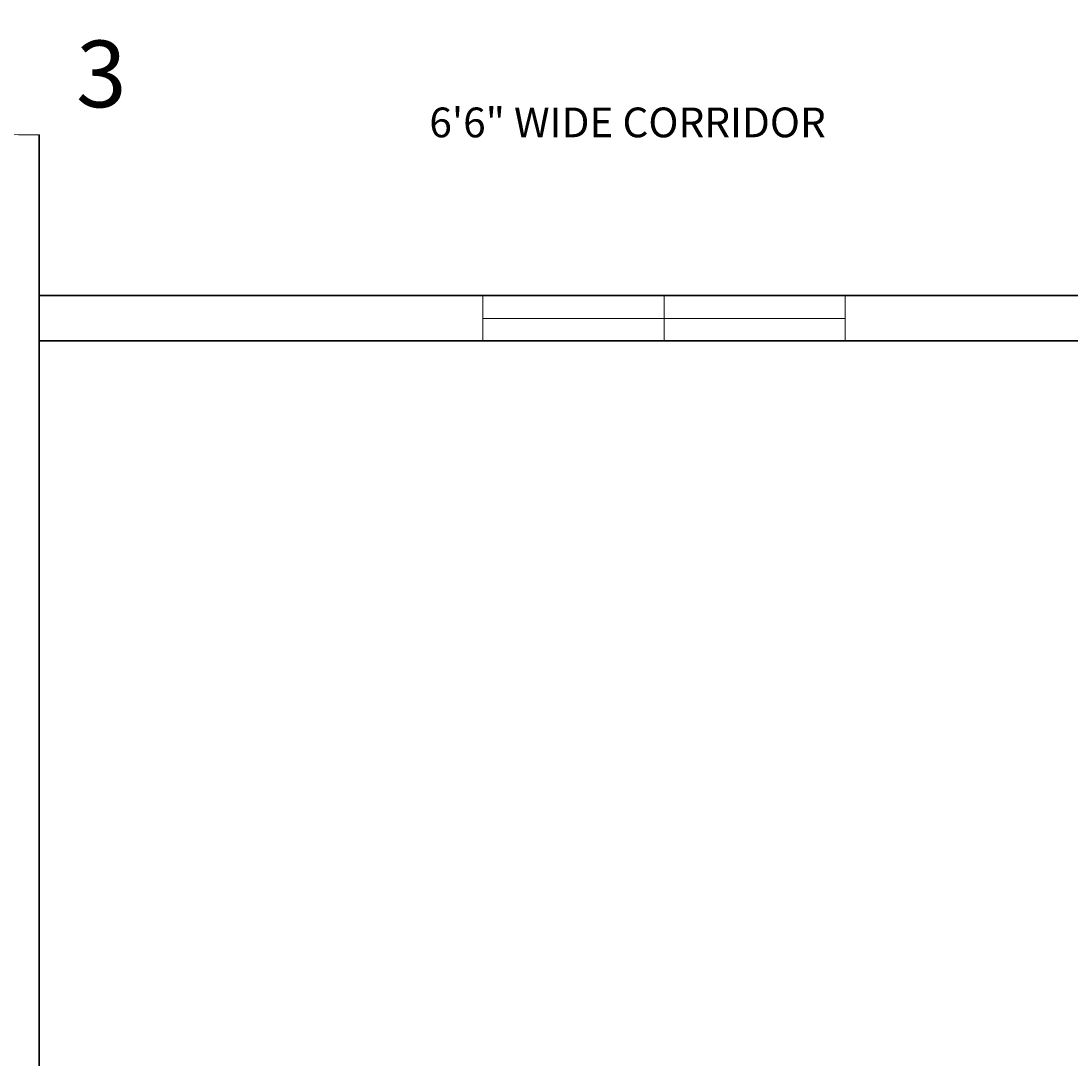
# Model space of a CAD drawing. Units: millimetres. Extents: x 27017497 to 27018854, y 7058029 to 7059154.
# Tile 59 of 91: x 27018038 to 27018246, y 7058203 to 7058409. Entities that reach past the tile are written whole.
import ezdxf

# ---------------------------------------------------------------- set-up
doc = ezdxf.new("R2010")
doc.units = ezdxf.units.MM
for name, color, linetype, lineweight in [('A-ANNO-DIMS', 2, 'Continuous', 18), ('A-ANNO-IDEN', 7, 'Continuous', 18), ('A-AREA-IDEN', 7, 'Continuous', 18), ('A-DOOR', 4, 'Continuous', 20), ('A-GLAZ', 4, 'Continuous', 18), ('A-WALL', 7, 'Continuous', 35)]:
    doc.layers.add(name, color=color, linetype=linetype, lineweight=lineweight)
doc.styles.get("Standard").update_dxf_attribs({"font": 'arial.ttf'})
doc.dimstyles.get("Standard").update_dxf_attribs({"dimtxt": 0.18, "dimasz": 0.18, "dimexe": 0.18, "dimexo": 0.0625, "dimgap": 0.09, "dimtad": 0, "dimtih": 1, "dimtoh": 1, "dimdec": 4, "dimzin": 0, "dimdsep": 46, "dimtxsty": 'Standard', "dimcen": 0.09, "dimadec": 0, "dimazin": 0, "dimtfac": 1, "dimtdec": 4, "dimtofl": 0, "dimtmove": 0, "dimatfit": 3, "dimfxl": 1, "dimtolj": 1, "dimtzin": 0, "dimarcsym": 0})

# ---------------------------------------------------------------- blocks, each defined once
blk = doc.blocks.new('*U2')
for p, q in [((0, 0), (0, -6)), ((40, 0), (40, -6))]:
    blk.add_line(p, q)
blk.add_lwpolyline([(0, 0), (0, 40), (1.75, 40), (1.75, 0)], close=True)
blk.add_arc((0, 0), 40, 0, 90)
blk = doc.blocks.new('WINDOW-SINGLE-LIGHT')
blk.add_lwpolyline([(36, 4.5), (36, 0), (0, 0), (0, 9), (36, 9), (36, 4.5), (0, 4.5)])
blk = doc.blocks.new('*D47')
at = {"layer": 'A-ANNO-DIMS', "color": 0, "lineweight": -2, "transparency": 16777216}
for p, q in [((27017561.17, 7058294.35), (27017561.17, 7058028.6)), ((27018790.61, 7058294.35), (27018790.61, 7058028.6)), ((27017561.35, 7058028.78), (27018175.43, 7058028.78)), ((27018790.43, 7058028.78), (27018176.34, 7058028.78))]:
    blk.add_line(p, q, dxfattribs=at)
at = {"layer": 'A-ANNO-DIMS', "color": 0, "transparency": 16777216}
for points in [[(27017561.35, 7058028.81), (27017561.35, 7058028.75), (27017561.17, 7058028.78)], [(27018790.43, 7058028.81), (27018790.43, 7058028.75), (27018790.61, 7058028.78)]]:
    blk.add_solid(points, dxfattribs=at)
at = {"layer": 'Defpoints', "color": 0, "transparency": 16777216}
for p in [(27017561.17, 7058294.41), (27018790.61, 7058294.41), (27018790.61, 7058028.78)]:
    blk.add_point(p, dxfattribs=at)
at = {"layer": 'A-ANNO-DIMS', "color": 0, "transparency": 16777216, "insert": (27018175.89, 7058028.78), "char_height": 0.18, "attachment_point": 5}
blk.add_mtext('\\A1;1229.4', dxfattribs=at)
blk = doc.blocks.new('*D48')
at = {"layer": 'A-ANNO-DIMS', "color": 0, "lineweight": -2, "transparency": 16777216}
for p, q in [((27018463.5, 7058622.91), (27017497.54, 7058622.91)), ((27017497.72, 7058622.73), (27017497.72, 7058357.75)), ((27017497.72, 7058092.41), (27017497.72, 7058357.39)), ((27018555.13, 7058092.23), (27017497.54, 7058092.23))]:
    blk.add_line(p, q, dxfattribs=at)
at = {"layer": 'A-ANNO-DIMS', "color": 0, "transparency": 16777216}
for points in [[(27017497.69, 7058622.73), (27017497.75, 7058622.73), (27017497.72, 7058622.91)], [(27017497.69, 7058092.41), (27017497.75, 7058092.41), (27017497.72, 7058092.23)]]:
    blk.add_solid(points, dxfattribs=at)
at = {"layer": 'Defpoints', "color": 0, "transparency": 16777216}
for p in [(27018463.56, 7058622.91), (27017497.72, 7058092.23), (27018555.19, 7058092.23)]:
    blk.add_point(p, dxfattribs=at)
at = {"layer": 'A-ANNO-DIMS', "color": 0, "transparency": 16777216, "insert": (27017497.72, 7058357.57), "char_height": 0.18, "attachment_point": 5}
blk.add_mtext('\\A1;530.7', dxfattribs=at)
blk = doc.blocks.new('*D51')
at = {"layer": 'A-ANNO-DIMS', "color": 0, "lineweight": -2, "transparency": 16777216}
for p, q in [((27018041.17, 7058345.35), (27018041.17, 7058028.6)), ((27018310.61, 7058345.35), (27018310.61, 7058028.6)), ((27018041.35, 7058028.78), (27018175.42, 7058028.78)), ((27018310.43, 7058028.78), (27018176.35, 7058028.78))]:
    blk.add_line(p, q, dxfattribs=at)
at = {"layer": 'A-ANNO-DIMS', "color": 0, "transparency": 16777216}
for points in [[(27018041.35, 7058028.81), (27018041.35, 7058028.75), (27018041.17, 7058028.78)], [(27018310.43, 7058028.81), (27018310.43, 7058028.75), (27018310.61, 7058028.78)]]:
    blk.add_solid(points, dxfattribs=at)
at = {"layer": 'Defpoints', "color": 0, "transparency": 16777216}
for p in [(27018041.17, 7058345.41), (27018310.61, 7058345.41), (27018310.61, 7058028.78)]:
    blk.add_point(p, dxfattribs=at)
at = {"layer": 'A-ANNO-DIMS', "color": 0, "transparency": 16777216, "insert": (27018175.89, 7058028.78), "char_height": 0.18, "attachment_point": 5}
blk.add_mtext('\\A1;269.44', dxfattribs=at)

msp = doc.modelspace()

# ---------------------------------------------------------------- linework, layer by layer
at = {"layer": 'A-WALL'}
for p, q in [((27018041.166, 7058386.357), (27018041.166, 7058375.363)), ((27018041.166, 7058386.357), (27018041.166, 7058246.045)), ((27018041.166, 7058386.357), (27018041.166, 7058132.912)), ((27018041.166, 7058354.412), (27018310.606, 7058354.412)), ((27018041.166, 7058345.412), (27018310.606, 7058345.412))]:
    msp.add_line(p, q, dxfattribs=at)

# ---------------------------------------------------------------- block references
at = {"layer": 'A-DOOR', "xscale": -0.6870473523349573, "yscale": 0.6870473523349573, "zscale": 0.6870473523349573, "rotation": 90}
msp.add_blockref('*U2', (27018037.095, 7058413.839), dxfattribs=at)
at = {"layer": 'A-GLAZ'}
for p in [(27018129.331, 7058345.371), (27018165.331, 7058345.371)]:
    msp.add_blockref('WINDOW-SINGLE-LIGHT', p, dxfattribs=at)

# ---------------------------------------------------------------- texts
at = {"layer": 'A-ANNO-IDEN'}
msp.add_text('3', height=13.242, dxfattribs=at).set_placement((27018048.518, 7058391.843))
at = {"layer": 'A-AREA-IDEN'}
msp.add_text('6\'6" WIDE CORRIDOR', height=5.91176, dxfattribs=at).set_placement((27018118.692, 7058385.868))

# ---------------------------------------------------------------- dimensions: what is measured, and where the dimension line sits
at = {"layer": 'A-ANNO-DIMS'}
dim = msp.add_linear_dim(base=(27017497.716, 7058092.23), p1=(27018463.561, 7058622.912), p2=(27018555.192, 7058092.23), angle=90, dimstyle='Standard', override={"dimdec": 1, "dimlfac": 1, "dimrnd": 0, "dimzin": 0, "dimdsep": 46, "dimlunit": 2}, dxfattribs=at)
dim.commit()
dim.dimension.update_dxf_attribs({"geometry": '*D48', "text_midpoint": (27017497.716, 7058357.571)})
for base, p1, p2, override, picture in [((27018310.606, 7058028.78), (27018041.166, 7058345.412), (27018310.606, 7058345.412), {"dimdec": 2, "dimlfac": 1, "dimrnd": 0, "dimzin": 0, "dimdsep": 46, "dimlunit": 2}, '*D51'), ((27018790.606, 7058028.78), (27017561.166, 7058294.412), (27018790.606, 7058294.412), {"dimdec": 1, "dimlfac": 1, "dimrnd": 0, "dimzin": 0, "dimdsep": 46, "dimlunit": 2}, '*D47')]:
    dim = msp.add_linear_dim(base=base, p1=p1, p2=p2, dimstyle='Standard', override=override, dxfattribs=at)
    dim.commit()
    dim.dimension.update_dxf_attribs({"geometry": picture, "text_midpoint": (27018175.886, 7058028.78)})

doc.saveas('drawing.dxf')
